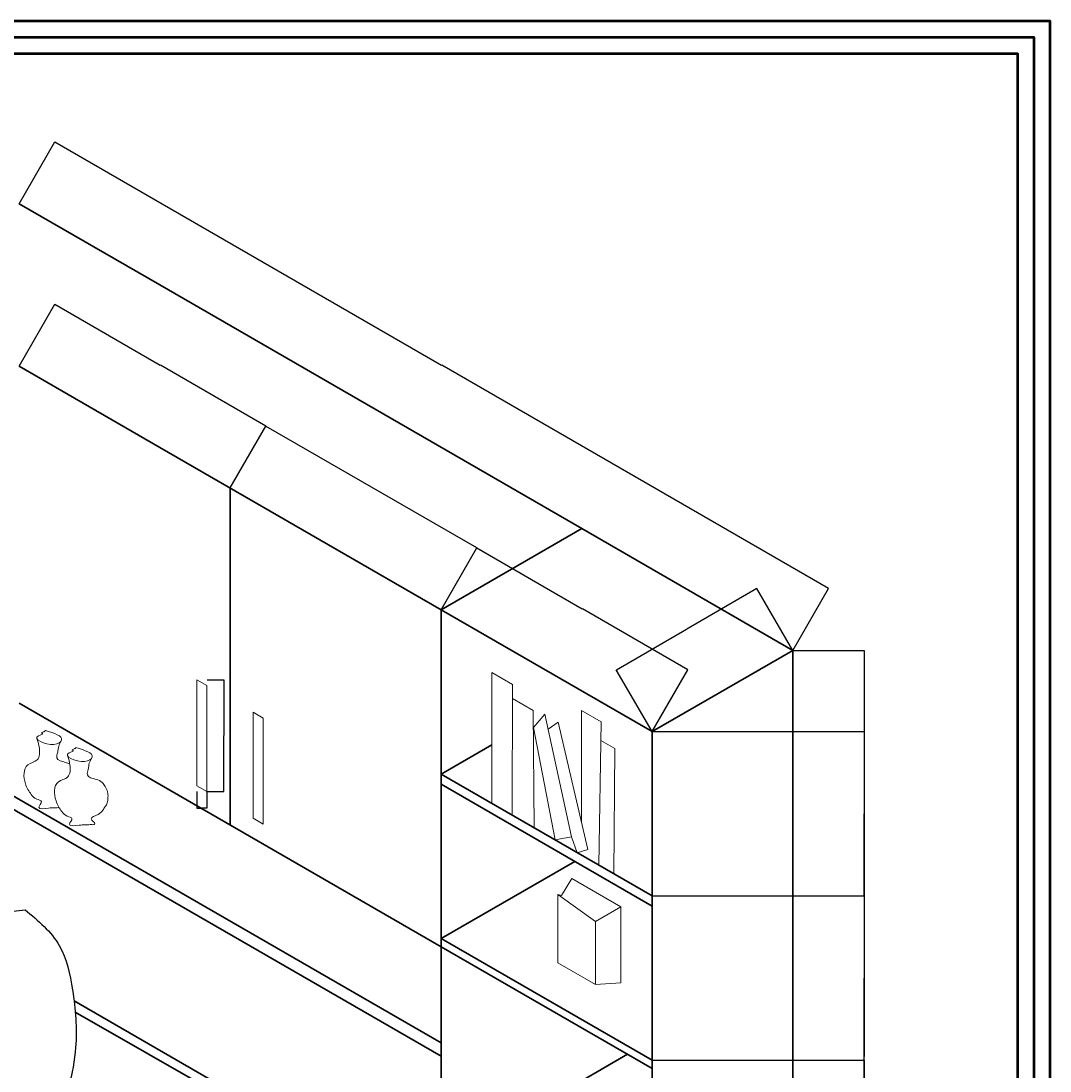
# Model space of a CAD drawing. Units: millimetres. Extents: x -2976 to 8877, y -7187 to 5690.
# Tile 2 of 2: x 2542 to 8877, y -776 to 5690. Entities that reach past the tile are written whole.
import ezdxf

# ---------------------------------------------------------------- set-up
doc = ezdxf.new("R2010")
doc.units = ezdxf.units.MM
doc.header["$MEASUREMENT"] = 0
for name, color, linetype, lineweight in [('A-ANNO-DIMS', 2, 'Continuous', 18), ('A-ANNO-TTLB', 7, 'Continuous', 50), ('A-FURN', 7, 'Continuous', 35), ('A-FURN-ACCS', 3, 'Continuous', 18), ('A-FURN-CHAIR', 4, 'Continuous', 25), ('A-FURN-HDWR', 8, 'Continuous', 18)]:
    doc.layers.add(name, color=color, linetype=linetype, lineweight=lineweight)
doc.styles.get("Standard").update_dxf_attribs({"font": 'arial.ttf'})
doc.dimstyles.get("Standard").update_dxf_attribs({"dimtxt": 0.18, "dimasz": 0.18, "dimexe": 0.18, "dimexo": 0.0625, "dimgap": 0.09, "dimtad": 0, "dimtih": 1, "dimtoh": 1, "dimdec": 0, "dimzin": 0, "dimdsep": 46, "dimtxsty": 'Standard', "dimcen": 0.09, "dimadec": 0, "dimazin": 0, "dimtfac": 1, "dimtdec": 0, "dimtofl": 0, "dimtmove": 0, "dimatfit": 3, "dimfxl": 1, "dimtolj": 1, "dimtzin": 0, "dimarcsym": 0})

# ---------------------------------------------------------------- blocks, each defined once
blk = doc.blocks.new('HANDLE-DOOR-R')
for p, q in [((8.8710727141e-05, 688.2438601006327), (8.8710727141e-05, 35.70737425468621)), ((8.8710727141e-05, 688.2438601006327), (61.8473034315216, 652.536354032953)), ((61.84730343152114, -0.0001318129926631), (61.8473034315216, 652.5363540329535)), ((8.8710727141e-05, 35.70737425468621), (61.84730343152114, -0.0001318129926631))]:
    blk.add_line(p, q)
blk = doc.blocks.new('*D11')
at = {"layer": 'A-ANNO-DIMS', "color": 0, "lineweight": -2, "transparency": 16777216}
for p, q in [((3687.362263616672, 1633.531567804586), (3790.716362403717, 1633.531567804586)), ((3790.536362403717, 1633.351567804586), (3790.536362403717, 1289.617627782288)), ((3790.536362403718, 945.4675758909599), (3790.536362403717, 1289.201515913257)), ((3687.362263616672, 945.28757589096), (3790.716362403717, 945.28757589096))]:
    blk.add_line(p, q, dxfattribs=at)
at = {"layer": 'A-ANNO-DIMS', "color": 0, "transparency": 16777216}
for points in [[(3790.506362403717, 1633.351567804586), (3790.566362403718, 1633.351567804586), (3790.536362403717, 1633.531567804586)], [(3790.506362403718, 945.4675758909599), (3790.566362403718, 945.4675758909599), (3790.536362403718, 945.28757589096)]]:
    blk.add_solid(points, dxfattribs=at)
at = {"layer": 'Defpoints', "color": 0, "transparency": 16777216}
for p in [(3687.299763616671, 1633.531567804586), (3790.536362403717, 1633.531567804586), (3687.299763616671, 945.28757589096)]:
    blk.add_point(p, dxfattribs=at)
at = {"layer": 'A-ANNO-DIMS', "color": 0, "transparency": 16777216, "insert": (3790.536362403717, 1289.409571847771), "char_height": 0.18, "attachment_point": 5}
blk.add_mtext('\\A1;DOOR HANDLE (RIGHT) 688 TYP.', dxfattribs=at)
blk = doc.blocks.new('*D12')
at = {"layer": 'A-ANNO-DIMS', "color": 0, "lineweight": -2, "transparency": 16777216}
for p, q in [((3625.452548895875, 945.2250758909595), (3625.452548895875, 841.870977103916)), ((3687.29976361667, 945.2250758909595), (3687.29976361667, 841.870977103916)), ((3625.632548895875, 842.0509771039158), (3655.847575083012, 842.0509771039158)), ((3687.11976361667, 842.0509771039158), (3656.904737429533, 842.0509771039158))]:
    blk.add_line(p, q, dxfattribs=at)
at = {"layer": 'A-ANNO-DIMS', "color": 0, "transparency": 16777216}
for points in [[(3625.632548895875, 842.0809771039158), (3625.632548895875, 842.0209771039159), (3625.452548895875, 842.0509771039158)], [(3687.11976361667, 842.0809771039158), (3687.11976361667, 842.0209771039159), (3687.29976361667, 842.0509771039158)]]:
    blk.add_solid(points, dxfattribs=at)
at = {"layer": 'Defpoints', "color": 0, "transparency": 16777216}
for p in [(3625.452548895875, 945.2875758909597), (3687.29976361667, 945.2875758909597), (3687.29976361667, 842.0509771039158)]:
    blk.add_point(p, dxfattribs=at)
at = {"layer": 'A-ANNO-DIMS', "color": 0, "transparency": 16777216, "insert": (3656.376156256273, 842.0509771039158), "char_height": 0.18, "attachment_point": 5}
blk.add_mtext('\\A1;62 TYP.', dxfattribs=at)
blk = doc.blocks.new('*D15')
at = {"layer": 'A-ANNO-DIMS', "color": 0, "lineweight": -2, "transparency": 16777216}
for p, q in [((7293.443979000004, 1814.359981000001), (7733.561479000008, 1814.359981000001)), ((7733.381479000008, 1814.179981000001), (7733.381479000008, -685.4581158622104)), ((7733.381479000008, -3185.460019000002), (7733.381479000008, -685.8219221377904)), ((7293.443979000004, -3185.640019000002), (7733.561479000008, -3185.640019000002))]:
    blk.add_line(p, q, dxfattribs=at)
at = {"layer": 'A-ANNO-DIMS', "color": 0, "transparency": 16777216}
for points in [[(7733.351479000008, 1814.179981000001), (7733.411479000007, 1814.179981000001), (7733.381479000008, 1814.359981000001)], [(7733.351479000008, -3185.460019000002), (7733.411479000007, -3185.460019000002), (7733.381479000008, -3185.640019000002)]]:
    blk.add_solid(points, dxfattribs=at)
at = {"layer": 'Defpoints', "color": 0, "transparency": 16777216}
for p in [(7293.381479000003, 1814.359981000001), (7293.381479000003, -3185.640019000002), (7733.381479000008, -3185.640019000002)]:
    blk.add_point(p, dxfattribs=at)
at = {"layer": 'A-ANNO-DIMS', "color": 0, "transparency": 16777216, "insert": (7733.381479000005, -685.6400190000024), "char_height": 0.18, "attachment_point": 5}
blk.add_mtext('\\A1;5000', dxfattribs=at)
blk = doc.blocks.new('*D26')
at = {"layer": 'A-ANNO-DIMS', "color": 0, "lineweight": -2, "transparency": 16777216}
for p, q in [((2530.273009, 4564.414107587735), (2750.331758610178, 4945.567042562642)), ((2750.397643182859, 4945.321157989961), (5131.496553235272, 3570.593061304077)), ((7513.225594241101, 2195.501158342615), (5132.126684188691, 3570.229255028497)), ((7293.412728999999, 1814.414107587736), (7513.471478813783, 2195.567042915297))]:
    blk.add_line(p, q, dxfattribs=at)
at = {"layer": 'A-ANNO-DIMS', "color": 0, "transparency": 16777216}
for points in [[(2750.412643182859, 4945.347138752074), (2750.382643182859, 4945.295177227848), (2750.241758610178, 4945.411157989961)], [(7513.240594241101, 2195.527139104729), (7513.210594241101, 2195.475177580502), (7513.381478813783, 2195.411158342615)]]:
    blk.add_solid(points, dxfattribs=at)
at = {"layer": 'Defpoints', "color": 0, "transparency": 16777216}
for p in [(2530.241759, 4564.359980999999), (7513.381478813783, 2195.411158342615), (7293.381479, 1814.359981)]:
    blk.add_point(p, dxfattribs=at)
at = {"layer": 'A-ANNO-DIMS', "color": 0, "transparency": 16777216, "insert": (5131.81161871198, 3570.411158166288), "char_height": 0.18, "attachment_point": 5}
blk.add_mtext('\\A1;5500', dxfattribs=at)
blk = doc.blocks.new('*D27')
at = {"layer": 'A-ANNO-DIMS', "color": 0, "lineweight": -2, "transparency": 16777216}
for p, q in [((7073.225594938394, 2195.321157779945), (6640.683843389727, 1945.593061087572)), ((7293.350228999999, 1814.414107587737), (7073.291479511074, 2195.567042352627)), ((6207.511960887646, 1695.501158119618), (6640.053712436311, 1945.229254811992)), ((6427.324825999999, 1314.414107587736), (6207.266076314964, 1695.567042692299))]:
    blk.add_line(p, q, dxfattribs=at)
at = {"layer": 'A-ANNO-DIMS', "color": 0, "transparency": 16777216}
for points in [[(7073.210594938394, 2195.347138542059), (7073.240594938394, 2195.295177017832), (7073.381479511074, 2195.411157779945)], [(6207.496960887645, 1695.527138881731), (6207.526960887646, 1695.475177357504), (6207.356076314964, 1695.411158119618)]]:
    blk.add_solid(points, dxfattribs=at)
at = {"layer": 'Defpoints', "color": 0, "transparency": 16777216}
for p in [(7073.381479511074, 2195.411157779945), (7293.381479, 1814.359981), (6427.356075999999, 1314.359980999999)]:
    blk.add_point(p, dxfattribs=at)
at = {"layer": 'A-ANNO-DIMS', "color": 0, "transparency": 16777216, "insert": (6640.368777913019, 1945.411157949781), "char_height": 0.18, "attachment_point": 5}
blk.add_mtext('\\A1;1000', dxfattribs=at)
blk = doc.blocks.new('*D29')
at = {"layer": 'A-ANNO-DIMS', "color": 0, "lineweight": -2, "transparency": 16777216}
for p, q in [((5128.34922, 2064.414107587737), (5348.407969752397, 2445.567042808975)), ((5348.473854325078, 2445.321158236293), (5997.521957235273, 2070.593061304076)), ((6647.200191098881, 1695.501158096281), (5998.15208818869, 2070.229255028495)), ((6427.387325999998, 1314.414107587737), (6647.446075671561, 1695.567042668963))]:
    blk.add_line(p, q, dxfattribs=at)
at = {"layer": 'A-ANNO-DIMS', "color": 0, "transparency": 16777216}
for points in [[(5348.488854325078, 2445.347138998406), (5348.458854325077, 2445.29517747418), (5348.317969752397, 2445.411158236293)], [(6647.215191098879, 1695.527138858394), (6647.185191098881, 1695.475177334168), (6647.356075671561, 1695.411158096281)]]:
    blk.add_solid(points, dxfattribs=at)
at = {"layer": 'Defpoints', "color": 0, "transparency": 16777216}
for p in [(5128.317970000001, 2064.359981), (6647.356075671561, 1695.411158096281), (6427.356075999999, 1314.359981)]:
    blk.add_point(p, dxfattribs=at)
at = {"layer": 'A-ANNO-DIMS', "color": 0, "transparency": 16777216, "insert": (5997.83702271198, 2070.411158166287), "char_height": 0.18, "attachment_point": 5}
blk.add_mtext('\\A1;1500', dxfattribs=at)
blk = doc.blocks.new('*D33')
at = {"layer": 'A-ANNO-DIMS', "color": 0, "lineweight": -2, "transparency": 16777216}
for p, q in [((2530.273009, 3564.414107587737), (2750.331758502398, 3945.567042375962)), ((2750.397643075079, 3945.321157803281), (3399.445745610272, 3570.593061087572)), ((4049.123979098881, 3195.501158096283), (3400.075876563688, 3570.229254811992)), ((3829.311114, 2814.414107587736), (4049.369863671563, 3195.567042668964))]:
    blk.add_line(p, q, dxfattribs=at)
at = {"layer": 'A-ANNO-DIMS', "color": 0, "transparency": 16777216}
for points in [[(2750.412643075078, 3945.347138565394), (2750.382643075079, 3945.295177041167), (2750.241758502398, 3945.411157803281)], [(4049.138979098881, 3195.527138858396), (4049.108979098881, 3195.47517733417), (4049.279863671563, 3195.411158096283)]]:
    blk.add_solid(points, dxfattribs=at)
at = {"layer": 'Defpoints', "color": 0, "transparency": 16777216}
for p in [(2530.241759, 3564.359981000001), (4049.279863671563, 3195.411158096283), (3829.279864, 2814.359981)]:
    blk.add_point(p, dxfattribs=at)
at = {"layer": 'A-ANNO-DIMS', "color": 0, "transparency": 16777216, "insert": (3399.76081108698, 3570.411157949782), "char_height": 0.18, "attachment_point": 5}
blk.add_mtext('\\A1;1500', dxfattribs=at)
blk = doc.blocks.new('*D34')
at = {"layer": 'A-ANNO-DIMS', "color": 0, "lineweight": -2, "transparency": 16777216}
for p, q in [((3829.311114, 2814.414107587737), (4049.369863752398, 3195.567042808975)), ((4049.435748325079, 3195.321158236294), (4698.483851235271, 2820.593061304078)), ((5348.162085098881, 2445.501158096283), (4699.113982188688, 2820.229255028499)), ((5128.34922, 2064.414107587737), (5348.407969671562, 2445.567042668964))]:
    blk.add_line(p, q, dxfattribs=at)
at = {"layer": 'A-ANNO-DIMS', "color": 0, "transparency": 16777216}
for points in [[(4049.450748325078, 3195.347138998407), (4049.420748325078, 3195.295177474181), (4049.279863752397, 3195.411158236294)], [(5348.177085098879, 2445.527138858396), (5348.14708509888, 2445.475177334169), (5348.317969671562, 2445.411158096283)]]:
    blk.add_solid(points, dxfattribs=at)
at = {"layer": 'Defpoints', "color": 0, "transparency": 16777216}
for p in [(3829.279864, 2814.359981), (5348.317969671562, 2445.411158096283), (5128.317970000001, 2064.359981)]:
    blk.add_point(p, dxfattribs=at)
at = {"layer": 'A-ANNO-DIMS', "color": 0, "transparency": 16777216, "insert": (4698.798916711979, 2820.411158166288), "char_height": 0.18, "attachment_point": 5}
blk.add_mtext('\\A1;1500', dxfattribs=at)
blk = doc.blocks.new('*D35')
at = {"layer": 'A-ANNO-DIMS', "color": 0, "lineweight": -2, "transparency": 16777216}
for p, q in [((6427.418576000004, 1314.359981), (7733.561479000008, 1314.359981000001)), ((7733.381479000008, 1314.179981000001), (7733.381479000008, 808.7530641377906)), ((7733.381479000008, 302.9623410000003), (7733.381479000008, 808.3892578622107)), ((6427.418576000004, 302.7823410000001), (7733.561479000008, 302.7823410000003))]:
    blk.add_line(p, q, dxfattribs=at)
at = {"layer": 'A-ANNO-DIMS', "color": 0, "transparency": 16777216}
for points in [[(7733.351479000008, 1314.179981000001), (7733.411479000007, 1314.179981000001), (7733.381479000008, 1314.359981000001)], [(7733.351479000008, 302.9623410000003), (7733.411479000007, 302.9623410000003), (7733.381479000008, 302.7823410000003)]]:
    blk.add_solid(points, dxfattribs=at)
at = {"layer": 'Defpoints', "color": 0, "transparency": 16777216}
for p in [(6427.356076000004, 1314.359981), (6427.356076000004, 302.7823410000001), (7733.381479000008, 302.7823410000003)]:
    blk.add_point(p, dxfattribs=at)
at = {"layer": 'A-ANNO-DIMS', "color": 0, "transparency": 16777216, "insert": (7733.381479000005, 808.5711609999983), "char_height": 0.18, "attachment_point": 5}
blk.add_mtext('\\A1;1011.6', dxfattribs=at)
blk = doc.blocks.new('*D36')
at = {"layer": 'A-ANNO-DIMS', "color": 0, "lineweight": -2, "transparency": 16777216}
for p, q in [((6427.418576000004, 302.7823410000001), (7733.561479000008, 302.7823410000003)), ((7733.381479000008, 302.6023410000003), (7733.381479000008, -203.3199808622101)), ((7733.381479000008, -709.6061090000001), (7733.381479000008, -203.6837871377898)), ((6427.418576000004, -709.7861090000002), (7733.561479000008, -709.7861090000001))]:
    blk.add_line(p, q, dxfattribs=at)
at = {"layer": 'A-ANNO-DIMS', "color": 0, "transparency": 16777216}
for points in [[(7733.351479000008, 302.6023410000003), (7733.411479000007, 302.6023410000003), (7733.381479000008, 302.7823410000003)], [(7733.351479000008, -709.6061090000001), (7733.411479000007, -709.6061090000001), (7733.381479000008, -709.7861090000001)]]:
    blk.add_solid(points, dxfattribs=at)
at = {"layer": 'Defpoints', "color": 0, "transparency": 16777216}
for p in [(6427.356076000004, 302.7823410000001), (6427.356076000004, -709.7861090000002), (7733.381479000008, -709.7861090000001)]:
    blk.add_point(p, dxfattribs=at)
at = {"layer": 'A-ANNO-DIMS', "color": 0, "transparency": 16777216, "insert": (7733.381479000005, -203.5018840000021), "char_height": 0.18, "attachment_point": 5}
blk.add_mtext('\\A1;1012.6', dxfattribs=at)
blk = doc.blocks.new('*D37')
at = {"layer": 'A-ANNO-DIMS', "color": 0, "lineweight": -2, "transparency": 16777216}
for p, q in [((6427.418576000004, -709.7861090000002), (7733.561479000008, -709.7861090000001)), ((7733.381479000008, -709.966109), (7733.381479000008, -1397.385788970669)), ((7733.381479000008, -2085.169398000001), (7733.381479000008, -1397.749718029332)), ((6427.418576000004, -2085.349398000001), (7733.561479000008, -2085.349398))]:
    blk.add_line(p, q, dxfattribs=at)
at = {"layer": 'A-ANNO-DIMS', "color": 0, "transparency": 16777216}
for points in [[(7733.351479000008, -709.966109), (7733.411479000007, -709.966109), (7733.381479000008, -709.7861090000001)], [(7733.351479000008, -2085.169398000001), (7733.411479000007, -2085.169398000001), (7733.381479000008, -2085.349398)]]:
    blk.add_solid(points, dxfattribs=at)
at = {"layer": 'Defpoints', "color": 0, "transparency": 16777216}
for p in [(6427.356076000004, -709.7861090000002), (6427.356076000004, -2085.349398000001), (7733.381479000008, -2085.349398)]:
    blk.add_point(p, dxfattribs=at)
at = {"layer": 'A-ANNO-DIMS', "color": 0, "transparency": 16777216, "insert": (7733.381479000005, -1397.567753500002), "char_height": 0.18, "attachment_point": 5}
blk.add_mtext('\\A1;1375.6', dxfattribs=at)

msp = doc.modelspace()

# ---------------------------------------------------------------- linework, layer by layer
at = {"layer": 'A-ANNO-TTLB'}
for points in [[(-2976.020185178524, 5689.883775799608), (8877.112005194242, 5689.883775799608), (8877.112005194242, -5692.972772104557), (-2976.020185178524, -5692.972772104557)], [(-2876.020185178524, 5589.883775799608), (8777.112005194242, 5589.883775799608), (8777.112005194242, -5592.972772104559), (-2876.020185178524, -5592.972772104556)], [(-2776.020185178524, 5489.883775799608), (8677.112005194242, 5489.883775799608), (8677.112005194242, -5492.972772104557), (-2776.020185178524, -5492.972772104557)]]:
    msp.add_lwpolyline(points, close=True, dxfattribs=at)
at = {"layer": 'A-FURN'}
for p, q in [((3396.267162442234, 4064.359980599718), (2530.241758657796, 4564.359980599717)), ((5994.343373795551, 2564.359980599718), (3396.267162442234, 4064.359980599718)), ((3396.267162442236, 3064.359980599719), (2530.241758657797, 3564.359980599719)), ((4955.112889254224, 2164.359980599719), (3396.267162442236, 3064.359980599719)), ((3829.279864334454, 739.842468911971), (3829.279864334454, 2814.35998059972)), ((5128.317970011113, 2064.359980599719), (5994.343373795551, 2564.359980599719)), ((7293.381479472209, 1814.35998059972), (5994.34337379555, 2564.359980599719)), ((5128.317970011113, 2064.359980599719), (4955.112889254224, 2164.359980599719)), ((6427.35607568777, 1314.359980599719), (5128.317970011113, 2064.359980599719)), ((5128.317970011113, 2064.359980599719), (5128.317970011111, -2935.640019400281)), ((7293.381479472209, -3185.640019400281), (7293.381479472209, 1814.35998059972)), ((5128.317970011113, -10.1575310880287), (2530.241758657797, 1489.842468911971)), ((6427.35607568777, -1085.64001940028), (6427.35607568777, 1314.359980599719)), ((5128.317970011113, 1052.782341466562), (5440.553578180447, 1233.051653893714)), ((5128.317970011113, 1052.782341466562), (6427.35607568777, 302.7823414665614)), ((5128.317970011113, 989.8836481307661), (6427.35607568777, 240.3570594793127)), ((5128.317970011113, -602.482296876944), (2461.912680004405, 936.9675150770705)), ((5128.317970011113, -683.3214143692167), (2462.198248141479, 855.963524743986)), ((5128.317970011113, 40.21389145139276), (5951.015754146192, 515.1986785834899)), ((5128.317970011113, 40.21389145139255), (6427.35607568777, -709.7861085486074)), ((5128.317970011113, -10.15753108802892), (6427.35607568777, -760.1575310880282)), ((5128.317970011111, -1648.386495488528), (2868.673209343396, -343.7799846440953)), ((2876.002629457045, -413.7919664145265), (5128.31797001111, -1699.325791095172)), ((5128.317970011111, -1335.349397541315), (6275.967791248173, -672.7534643146713))]:
    msp.add_line(p, q, dxfattribs=at)
msp.add_lwpolyline([(6427.35607568777, 1314.359980599719), (7293.381479472209, 1814.359980599719)], dxfattribs=at)
at = {"layer": 'A-FURN-ACCS'}
for p, q in [((5440.921041696739, 1677.213208936606), (5440.255439951728, 872.685159226016)), ((5440.921041696739, 1677.213208936606), (5567.506460965553, 1604.129083046275)), ((5567.506460965553, 1604.129083046275), (5566.18919161124, 799.9772738053377)), ((5567.36509349384, 1517.828655747072), (5696.174829426658, 1443.460320032015)), ((5696.174829426658, 1443.460320032015), (5702.307965889136, 721.389062834232)), ((5993.740641487093, 1444.247379130771), (5991.882106086484, 758.7770641425227)), ((5993.740641487093, 1444.247379130771), (6114.162973225116, 1374.721513485381)), ((5766.915290812809, 1421.476676535194), (5697.060181220925, 1339.22538460218)), ((5931.469937127476, 666.692940264118), (5766.915290812809, 1421.476676535194)), ((5786.953522166026, 1329.564770868772), (5849.187271530565, 1372.400718487944)), ((5849.187271530565, 1372.400718487944), (6031.636095271591, 587.8249186462198)), ((6114.162973225116, 1374.721513485381), (6100.541433646729, 491.4688630240678)), ((5697.060181220925, 1339.22538460218), (5830.748002831144, 647.2341729310388)), ((6112.381190533181, 1259.186534774542), (6197.53222456231, 1210.02456235605)), ((6197.53222456231, 1210.02456235605), (6192.463498029229, 438.3976344083658)), ((5830.748002831144, 647.2341729310388), (5931.469937127476, 666.692940264118)), ((5967.109209518468, 568.5059935430902), (5931.469937127476, 666.692940264118)), ((6031.636095271591, 587.8249186462198), (5967.109209518468, 568.5059935430902)), ((5933.523154944676, 408.7332978922484), (5869.657758955291, 304.1966358796921)), ((6235.261028794105, 234.5248552005758), (5933.523154944676, 408.7332978922484)), ((5846.357046359102, 310.2796607425407), (5846.357046359102, -108.6022311681232)), ((5869.657758955291, 304.1966358796923), (5846.357046359102, 310.2796607425407)), ((5846.357046359102, 310.2796607425407), (6078.927086429991, 144.2654114931793)), ((6078.927086429991, 144.2654114931793), (6235.261028794105, 234.5248552005758)), ((6235.261028794105, 234.5248552005758), (6235.261028794105, -232.4965489628705)), ((6078.927086429991, -242.8766064084927), (6078.927086429992, 144.2654114931787)), ((5846.357046359102, -108.6022311681232), (6078.927086429991, -242.8766064084927)), ((6235.261028794105, -232.4965489628705), (6078.927086429991, -242.8766064084927))]:
    msp.add_line(p, q, dxfattribs=at)
for points, knots in [([(2692.523164543032, 1320.63690926609), (2746.212604694743, 1304.047594083937), (2825.881690888548, 1279.430917556699), (2736.503026892276, 1210.803761117802), (2585.067620712597, 1278.205472364463), (2685.998169374182, 1298.989460134514), (2662.918202765178, 1307.09250964623), (2678.866955921248, 1311.015754532864), (2684.818756584213, 1314.994835207012), (2689.159207544991, 1316.904499837071), (2691.472965576529, 1319.471682562179), (2692.523164543032, 1320.63690926609)], [0, 0, 0, 0, 115.4373651336158, 171.2960568563994, 279.0731841669098, 306.4387679226323, 312.7692218456463, 327.1537514953741, 330.4307730061897, 336.0614474905891, 340.7413462684733, 340.7413462684733, 340.7413462684733, 340.7413462684733]), ([(2642.746906646784, 1266.139652301674), (2647.695506745537, 1249.416448545932), (2659.468926767118, 1209.629579937895), (2657.716786505414, 1129.957126922568), (2552.97477879331, 1115.627763633366), (2558.075726327194, 999.8327569732583), (2598.04641180261, 934.1266305384316), (2629.857801635824, 897.2954305183538), (2684.274507467886, 888.5516725699005), (2626.461016420487, 831.4478408651602), (2708.622104245675, 843.1239916198306), (2741.710149426291, 846.0352679658537), (2764.277582288048, 845.1603331563482), (2774.54363836981, 846.753852448739), (2776.508579985107, 847.029482080743)], [0, 0, 0, 0, 53.89871295787923, 128.2326665344357, 194.6274369626239, 311.0043774434725, 386.3724247320341, 430.2818943451568, 463.101306931476, 501.2731315190478, 561.6183083840479, 595.0182481110646, 620.3011744944619, 626.2879899616084, 626.2879899616084, 626.2879899616084, 626.2879899616084]), ([(2842.597476619524, 1114.885498834935), (2834.881176341094, 1119.156905302542), (2806.237565920907, 1128.522765818416), (2751.849904857971, 1139.950728446129), (2771.034694948802, 1189.061173670217), (2770.908385693303, 1224.83465270344), (2783.850236372932, 1247.030850339889), (2790.167744979405, 1257.86582851036)], [991.4852151599173, 991.4852151599173, 991.4852151599173, 991.4852151599173, 1018.898613637143, 1078.679283416861, 1113.127763885908, 1151.570490271903, 1188.232584728662, 1188.232584728662, 1188.232584728662, 1188.232584728662]), ([(2880.773360913765, 1215.602798501451), (2934.462801065476, 1199.013483319298), (3014.131887259281, 1174.396806792061), (2924.753223263008, 1105.769650353163), (2773.317817083332, 1173.171361599825), (2874.248365744914, 1193.955349369876), (2851.168399135911, 1202.058398881592), (2867.117152291981, 1205.981643768226), (2873.068952954946, 1209.960724442374), (2877.409403915724, 1211.870389072432), (2879.723161947262, 1214.437571797541), (2880.773360913765, 1215.602798501451)], [0, 0, 0, 0, 115.4373651336158, 171.2960568563994, 279.0731841669098, 306.4387679226323, 312.7692218456463, 327.1537514953741, 330.4307730061897, 336.0614474905891, 340.7413462684733, 340.7413462684733, 340.7413462684733, 340.7413462684733]), ([(2830.997103017517, 1161.105541537035), (2835.94570311627, 1144.382337781294), (2847.71912313785, 1104.595469173258), (2845.966982876147, 1024.923016157929), (2741.224975164041, 1010.593652868728), (2746.325922697929, 894.79864620862), (2786.296608173343, 829.0925197737934), (2818.107998006555, 792.2613197537158), (2872.524703838618, 783.5175618052625), (2814.71121279122, 726.4137301005218), (2896.872300616407, 738.0898808551923), (2929.960345797024, 741.0011572012152), (2957.123646518812, 739.9480415239411), (2975.862994307004, 744.5285364828483), (2991.00991582088, 737.87673006034), (2999.399233865915, 750.2005147605923), (2985.420724339046, 761.2517412046509), (2959.829553119368, 786.7279497508713), (3019.066893241068, 800.7952260399034), (3045.033281611953, 824.7780394380954), (3056.162423820392, 849.7255197529424), (3071.391414809758, 866.4388370741709), (3076.404627951844, 887.8234969073435), (3078.380718860223, 914.1648561374324), (3077.77049076669, 944.8852388650122), (3060.73490448118, 973.7448634183218), (3042.407661715744, 1007.397105074166), (3001.286819592389, 1022.060033722798), (2940.100101228705, 1034.916617681491), (2959.284891319534, 1084.027062905579), (2959.158582064037, 1119.800541938801), (2972.100432743665, 1141.996739575251), (2978.417941350138, 1152.831717745722)], [0, 0, 0, 0, 53.89871295787923, 128.2326665344357, 194.6274369626239, 311.0043774434725, 386.3724247320341, 430.2818943451568, 463.101306931476, 501.2731315190478, 561.6183083840479, 595.0182481110646, 620.3011744944619, 639.457999723088, 653.6509631414006, 661.6430805440533, 674.3553248466898, 699.0572658528314, 749.3411743416673, 788.6813671985493, 813.4254089212131, 828.7808019033675, 855.8036652260705, 876.5297583894804, 908.9375671083436, 945.0916138557602, 976.2785553618417, 1018.898613637143, 1078.679283416861, 1113.127763885908, 1151.570490271903, 1188.232584728662, 1188.232584728662, 1188.232584728662, 1188.232584728662])]:
    msp.add_open_spline(points, degree=3, knots=knots, dxfattribs=at)
at = {"layer": 'A-FURN-CHAIR'}
msp.add_open_spline([(2567.327213554687, 217.3777815164612), (2371.604006962237, 192.7327323130228), (2081.31339379434, 156.1799567409558), (2150.139936282865, -182.4667104222866), (2165.116014388808, -365.952377867469), (2201.134482322425, -570.5848202688835), (2001.966179159994, -713.9202466194699), (1796.942794050407, -716.3269363524186), (1590.45379523456, -678.4075351907952), (1425.098437734223, -813.6407202142198), (1195.207760947901, -994.0076673186782), (1334.194099928929, -1211.943894338208), (1433.600624954212, -1310.666009676965), (1490.614413886304, -1345.956672059368), (1614.157571527384, -1391.232703225471), (1813.084480556488, -1488.982700143385), (2144.550172737321, -1441.760630520553), (2511.026644645633, -1393.796613114915), (2787.65137241148, -1067.523731355003), (2900.240674189164, -675.4125804627595), (2869.868896878056, -301.0233351137475), (2802.881672971835, 19.87963263450726), (2647.650590440668, 150.0314944362605), (2567.327213554687, 217.3777815164612)], degree=3, knots=[0, 0, 0, 0, 465.8253811586821, 690.8978137033012, 888.5150348665003, 1055.970420950123, 1257.901159625074, 1514.322789017122, 1677.169158812602, 1848.867129305455, 2138.548569140127, 2410.457651988302, 2465.321249117196, 2565.415027162817, 2606.552378177621, 2860.949289062645, 3210.570075939517, 3586.794658316177, 3928.74340176956, 4419.123148240912, 4773.689233456088, 5058.287964198188, 5363.462590944195, 5363.462590944195, 5363.462590944195, 5363.462590944195], dxfattribs=at)

# ---------------------------------------------------------------- block references
at = {"layer": 'A-FURN-HDWR'}
for p in [(3625.452460185148, 945.2877077039524), (3972.018, 745.1979999999999)]:
    msp.add_blockref('HANDLE-DOOR-R', p, dxfattribs=at)

# ---------------------------------------------------------------- dimensions: what is measured, and where the dimension line sits
at = {"layer": 'A-ANNO-DIMS'}
for base, p1, p2, angle, override, picture, middle in [((7513.381478813783, 2195.411158342615), (2530.241759, 4564.359980999999), (7293.381479, 1814.359981), 330.0000000000001, {"dimdec": 0, "dimlfac": 1, "dimrnd": 0, "dimzin": 0, "dimdsep": 46, "dimlunit": 2}, '*D26', (5131.81161871198, 3570.411158166288)), ((4049.279863671563, 3195.411158096283), (2530.241759, 3564.359981000001), (3829.279864, 2814.359981), 330.0000000000001, {"dimdec": 0, "dimlfac": 1, "dimrnd": 0, "dimzin": 0, "dimdsep": 46, "dimlunit": 2}, '*D33', (3399.76081108698, 3570.411157949782)), ((5348.317969671562, 2445.411158096283), (3829.279864, 2814.359981), (5128.317970000001, 2064.359981), 330, {"dimdec": 0, "dimlfac": 1, "dimrnd": 0, "dimzin": 0, "dimdsep": 46, "dimlunit": 2}, '*D34', (4698.798916711979, 2820.411158166288)), ((6647.356075671561, 1695.411158096281), (5128.317970000001, 2064.359981), (6427.356075999999, 1314.359981), 330, {"dimdec": 0, "dimlfac": 1, "dimrnd": 0, "dimzin": 0, "dimdsep": 46, "dimlunit": 2}, '*D29', (5997.83702271198, 2070.411158166287)), ((7073.381479511074, 2195.411157779945), (6427.356075999999, 1314.359981), (7293.381479, 1814.359981), 29.99999999999997, {"dimdec": 0, "dimlfac": 1, "dimrnd": 0, "dimzin": 0, "dimdsep": 46, "dimlunit": 2}, '*D27', (6640.368777913019, 1945.411157949781)), ((7733.381479000008, -3185.640019000002), (7293.381479, 1814.359981), (7293.381479, -3185.640019), 90, {"dimdec": 0, "dimlfac": 1, "dimrnd": 0, "dimzin": 0, "dimdsep": 46, "dimlunit": 2}, '*D15', (7733.381479000005, -685.6400190000024)), ((7733.381479000008, 302.7823410000003), (6427.356075999999, 1314.359981), (6427.356075999999, 302.782341), 90, {"dimdec": 1, "dimlfac": 1, "dimrnd": 0, "dimzin": 0, "dimdsep": 46, "dimlunit": 2}, '*D35', (7733.381479000005, 808.5711609999983)), ((7733.381479000008, -709.7861090000001), (6427.356075999999, 302.782341), (6427.356075999999, -709.786109), 90, {"dimdec": 1, "dimlfac": 1, "dimrnd": 0, "dimzin": 0, "dimdsep": 46, "dimlunit": 2}, '*D36', (7733.381479000005, -203.5018840000021)), ((7733.381479000008, -2085.349398), (6427.356075999999, -709.786109), (6427.356075999999, -2085.349398), 90, {"dimdec": 1, "dimlfac": 1, "dimrnd": 0, "dimzin": 0, "dimdsep": 46, "dimlunit": 2}, '*D37', (7733.381479000005, -1397.567753500002))]:
    dim = msp.add_linear_dim(base=base, p1=p1, p2=p2, angle=angle, dimstyle='Standard', override=override, dxfattribs=at)
    dim.commit()
    dim.dimension.update_dxf_attribs({"geometry": picture, "text_midpoint": middle})
dim = msp.add_linear_dim(base=(3790.536362403717, 1633.531567804586), p1=(3687.29976361667, 945.2875758909597), p2=(3687.29976361667, 1633.531567804585), angle=90, text='DOOR HANDLE (RIGHT) <> TYP.', dimstyle='Standard', override={"dimdec": 0, "dimlfac": 1, "dimrnd": 0, "dimzin": 0, "dimdsep": 46, "dimlunit": 2}, dxfattribs=at)
dim.commit()
dim.dimension.update_dxf_attribs({"geometry": '*D11', "text_midpoint": (3790.536362403717, 1289.409571847771)})
dim = msp.add_linear_dim(base=(3687.29976361667, 842.0509771039158), p1=(3625.452548895875, 945.2875758909597), p2=(3687.29976361667, 945.2875758909597), text='<> TYP.', dimstyle='Standard', override={"dimdec": 0, "dimlfac": 1, "dimrnd": 0, "dimzin": 0, "dimdsep": 46, "dimlunit": 2}, dxfattribs=at)
dim.commit()
dim.dimension.update_dxf_attribs({"geometry": '*D12', "text_midpoint": (3656.376156256273, 842.0509771039158)})

doc.saveas('drawing.dxf')
